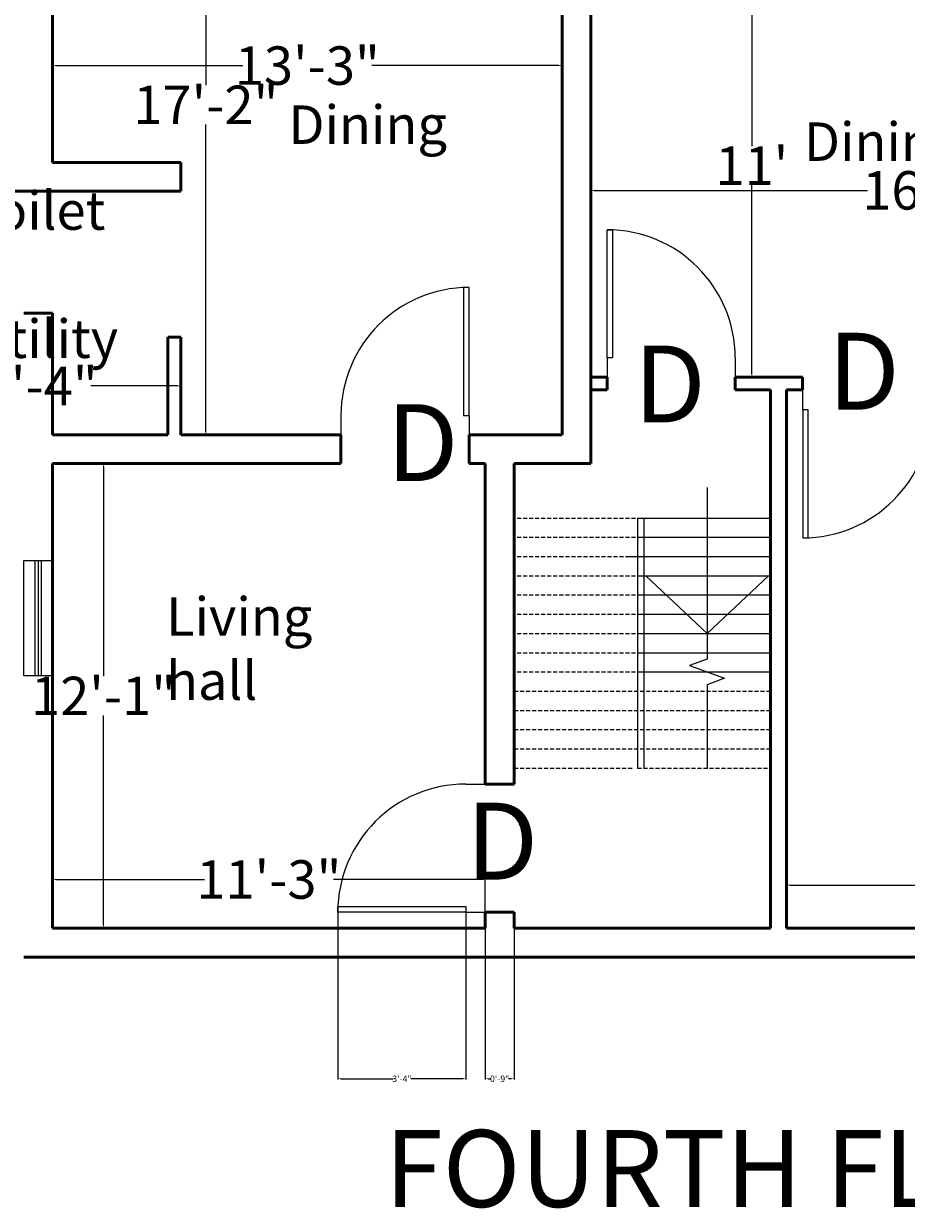
# Model space of a CAD drawing. Units: inches. Extents: x 409 to 7572, y 7 to 725.
# Tile 28 of 38: x 5677 to 5952, y 78 to 448. Entities that reach past the tile are written whole.
import ezdxf

# ---------------------------------------------------------------- set-up
doc = ezdxf.new("R2010")
doc.units = ezdxf.units.IN
doc.header["$MEASUREMENT"] = 0
doc.linetypes.add('HIDDEN', pattern=[0.375, 0.25, -0.125])
for name, color, linetype, lineweight in [('A-ANNO-DIMS', 2, 'Continuous', 18), ('A-ANNO-SYMB', 3, 'Continuous', 25), ('A-ANNO-TEXT', 7, 'Continuous', 35), ('A-AREA-IDEN', 7, 'Continuous', 25), ('A-DOOR', 3, 'Continuous', 25), ('A-FLOR-STRS', 6, 'Continuous', 25), ('A-FLOR-STRS-OVHD', 6, 'HIDDEN', 18), ('A-GLAZ', 4, 'Continuous', 25), ('A-WALL', 7, 'Continuous', 50)]:
    doc.layers.add(name, color=color, linetype=linetype, lineweight=lineweight)
doc.styles.get("Standard").update_dxf_attribs({"font": 'arial.ttf'})
doc.dimstyles.get("Standard").update_dxf_attribs({"dimtxt": 2, "dimasz": 1, "dimexe": 0.18, "dimexo": 0.0625, "dimgap": 0.09, "dimtad": 0, "dimtih": 1, "dimtoh": 1, "dimdec": 0, "dimzin": 0, "dimdsep": 46, "dimlunit": 3, "dimtxsty": 'Standard', "dimcen": 0.09, "dimadec": 0, "dimazin": 0, "dimtfac": 1, "dimtdec": 0, "dimtofl": 0, "dimtmove": 0, "dimatfit": 3, "dimfxl": 1, "dimtolj": 1, "dimtzin": 0, "dimarcsym": 0})

# ---------------------------------------------------------------- blocks, each defined once
blk = doc.blocks.new('*U2')
for p, q in [((0, 0), (0, -6)), ((-40, 0), (-40, -6))]:
    blk.add_line(p, q)
blk.add_lwpolyline([(0, 0), (0, 40), (-1.75, 40), (-1.75, 0)], close=True)
blk.add_arc((0, 0), 40, 90, 180)
blk = doc.blocks.new('*U3')
for p, q in [((0, 0), (0, -6)), ((40, 0), (40, -6))]:
    blk.add_line(p, q)
blk.add_lwpolyline([(0, 0), (0, 40), (1.75, 40), (1.75, 0)], close=True)
blk.add_arc((0, 0), 40, 0, 90)
blk = doc.blocks.new('*U4')
for p, q in [((0, 0), (0, -6)), ((40, 0), (40, -6))]:
    blk.add_line(p, q)
blk.add_lwpolyline([(0, 0), (0, 40), (1.75, 40), (1.75, 0)], close=True)
blk.add_arc((0, 0), 40, 0, 90)
blk = doc.blocks.new('*U5')
for p, q in [((0, 0), (0, 6)), ((40, 0), (40, 6))]:
    blk.add_line(p, q)
blk.add_lwpolyline([(0, 0), (0, -40), (1.75, -40), (1.75, 0)], close=True)
blk.add_arc((0, 0), 40, 270, 0)
blk = doc.blocks.new('*D124')
at = {"layer": 'A-ANNO-DIMS', "color": 0, "lineweight": -2, "transparency": 16777216}
for p, q in [((5914.78, 165.59), (5914.78, 179.18)), ((5915.78, 179), (5962.65, 179)), ((6049.78, 179), (6002.92, 179)), ((6050.78, 165.59), (6050.78, 179.18))]:
    blk.add_line(p, q, dxfattribs=at)
at = {"layer": 'A-ANNO-DIMS', "color": 0, "transparency": 16777216}
for points in [[(5915.78, 179.16), (5915.78, 178.83), (5914.78, 179)], [(6049.78, 179.16), (6049.78, 178.83), (6050.78, 179)]]:
    blk.add_solid(points, dxfattribs=at)
at = {"layer": 'DEFPOINTS', "color": 0, "transparency": 16777216}
for p in [(6050.78, 179), (5914.78, 165.53), (6050.78, 165.53)]:
    blk.add_point(p, dxfattribs=at)
at = {"layer": 'A-ANNO-DIMS', "color": 0, "transparency": 16777216, "insert": (5982.78, 179), "char_height": 2, "attachment_point": 5}
blk.add_mtext('\\A1;{\\H6x;11\'-4"}', dxfattribs=at)
blk = doc.blocks.new('*D125')
at = {"layer": 'A-ANNO-DIMS', "color": 0, "lineweight": -2, "transparency": 16777216}
for p, q in [((5685.78, 165.59), (5685.78, 180.91)), ((5686.78, 180.73), (5733.15, 180.73)), ((5819.78, 180.73), (5773.42, 180.73)), ((5820.78, 165.59), (5820.78, 180.91))]:
    blk.add_line(p, q, dxfattribs=at)
at = {"layer": 'A-ANNO-DIMS', "color": 0, "transparency": 16777216}
for points in [[(5686.78, 180.9), (5686.78, 180.56), (5685.78, 180.73)], [(5819.78, 180.9), (5819.78, 180.56), (5820.78, 180.73)]]:
    blk.add_solid(points, dxfattribs=at)
at = {"layer": 'DEFPOINTS', "color": 0, "transparency": 16777216}
for p in [(5820.78, 180.73), (5685.78, 165.53), (5820.78, 165.53)]:
    blk.add_point(p, dxfattribs=at)
at = {"layer": 'A-ANNO-DIMS', "color": 0, "transparency": 16777216, "insert": (5753.28, 180.73), "char_height": 2, "attachment_point": 5}
blk.add_mtext('\\A1;{\\H6x;11\'-3"}', dxfattribs=at)
blk = doc.blocks.new('*D126')
at = {"layer": 'A-ANNO-DIMS', "color": 0, "lineweight": -2, "transparency": 16777216}
for p, q in [((5685.85, 310.53), (5701.89, 310.53)), ((5701.71, 309.53), (5701.71, 244.15)), ((5701.71, 166.53), (5701.71, 231.92)), ((5685.85, 165.53), (5701.89, 165.53))]:
    blk.add_line(p, q, dxfattribs=at)
at = {"layer": 'A-ANNO-DIMS', "color": 0, "transparency": 16777216}
for points in [[(5701.54, 309.53), (5701.87, 309.53), (5701.71, 310.53)], [(5701.54, 166.53), (5701.87, 166.53), (5701.71, 165.53)]]:
    blk.add_solid(points, dxfattribs=at)
at = {"layer": 'DEFPOINTS', "color": 0, "transparency": 16777216}
for p in [(5685.78, 310.53), (5685.78, 165.53), (5701.71, 165.53)]:
    blk.add_point(p, dxfattribs=at)
at = {"layer": 'A-ANNO-DIMS', "color": 0, "transparency": 16777216, "insert": (5701.71, 238.03), "char_height": 2, "attachment_point": 5}
blk.add_mtext('\\A1;{\\H6x;12\'-1"}', dxfattribs=at)
blk = doc.blocks.new('*D138')
at = {"layer": 'A-ANNO-DIMS', "color": 0, "lineweight": -2, "transparency": 16777216}
for p, q in [((5685.78, 404.59), (5685.78, 434.95)), ((5686.78, 434.77), (5745.15, 434.77)), ((5843.78, 434.77), (5785.42, 434.77)), ((5844.78, 404.59), (5844.78, 434.95))]:
    blk.add_line(p, q, dxfattribs=at)
at = {"layer": 'A-ANNO-DIMS', "color": 0, "transparency": 16777216}
for points in [[(5686.78, 434.93), (5686.78, 434.6), (5685.78, 434.77)], [(5843.78, 434.93), (5843.78, 434.6), (5844.78, 434.77)]]:
    blk.add_solid(points, dxfattribs=at)
at = {"layer": 'DEFPOINTS', "color": 0, "transparency": 16777216}
for p in [(5844.78, 434.77), (5685.78, 404.53), (5844.78, 404.53)]:
    blk.add_point(p, dxfattribs=at)
at = {"layer": 'A-ANNO-DIMS', "color": 0, "transparency": 16777216, "insert": (5765.28, 434.77), "char_height": 2, "attachment_point": 5}
blk.add_mtext('\\A1;{\\H6x;13\'-3"}', dxfattribs=at)
blk = doc.blocks.new('*D139')
at = {"layer": 'A-ANNO-DIMS', "color": 0, "lineweight": -2, "transparency": 16777216}
for p, q in [((5742.72, 525.53), (5733.44, 525.53)), ((5733.62, 524.53), (5733.62, 428.65)), ((5733.62, 320.53), (5733.62, 416.42)), ((5750.72, 319.53), (5733.44, 319.53))]:
    blk.add_line(p, q, dxfattribs=at)
at = {"layer": 'A-ANNO-DIMS', "color": 0, "transparency": 16777216}
for points in [[(5733.45, 524.53), (5733.79, 524.53), (5733.62, 525.53)], [(5733.45, 320.53), (5733.79, 320.53), (5733.62, 319.53)]]:
    blk.add_solid(points, dxfattribs=at)
at = {"layer": 'DEFPOINTS', "color": 0, "transparency": 16777216}
for p in [(5742.78, 525.53), (5733.62, 319.53), (5750.78, 319.53)]:
    blk.add_point(p, dxfattribs=at)
at = {"layer": 'A-ANNO-DIMS', "color": 0, "transparency": 16777216, "insert": (5733.62, 422.53), "char_height": 2, "attachment_point": 5}
blk.add_mtext('\\A1;{\\H6x;17\'-2"}', dxfattribs=at)
blk = doc.blocks.new('*D136')
at = {"layer": 'A-ANNO-DIMS', "color": 0, "lineweight": -2, "transparency": 16777216}
for p, q in [((5853.78, 403.47), (5853.78, 395.65)), ((6045.78, 403.47), (6045.78, 395.65)), ((5854.78, 395.83), (5940.08, 395.83)), ((6044.78, 395.83), (5959.49, 395.83))]:
    blk.add_line(p, q, dxfattribs=at)
at = {"layer": 'A-ANNO-DIMS', "color": 0, "transparency": 16777216}
for points in [[(5854.78, 396), (5854.78, 395.66), (5853.78, 395.83)], [(6044.78, 396), (6044.78, 395.66), (6045.78, 395.83)]]:
    blk.add_solid(points, dxfattribs=at)
at = {"layer": 'DEFPOINTS', "color": 0, "transparency": 16777216}
for p in [(5853.78, 403.53), (6045.78, 403.53), (6045.78, 395.83)]:
    blk.add_point(p, dxfattribs=at)
at = {"layer": 'A-ANNO-DIMS', "color": 0, "transparency": 16777216, "insert": (5949.78, 395.83), "char_height": 2, "attachment_point": 5}
blk.add_mtext("\\A1;{\\H6x;16'}", dxfattribs=at)
blk = doc.blocks.new('*D140')
at = {"layer": 'A-ANNO-DIMS', "color": 0, "lineweight": -2, "transparency": 16777216}
for p, q in [((5908.05, 469.53), (5903.8, 469.53)), ((5903.98, 468.53), (5903.98, 409.65)), ((5903.98, 338.53), (5903.98, 397.42)), ((5909.22, 337.53), (5903.8, 337.53))]:
    blk.add_line(p, q, dxfattribs=at)
at = {"layer": 'A-ANNO-DIMS', "color": 0, "transparency": 16777216}
for points in [[(5903.81, 468.53), (5904.15, 468.53), (5903.98, 469.53)], [(5903.81, 338.53), (5904.15, 338.53), (5903.98, 337.53)]]:
    blk.add_solid(points, dxfattribs=at)
at = {"layer": 'DEFPOINTS', "color": 0, "transparency": 16777216}
for p in [(5908.11, 469.53), (5903.98, 337.53), (5909.28, 337.53)]:
    blk.add_point(p, dxfattribs=at)
at = {"layer": 'A-ANNO-DIMS', "color": 0, "transparency": 16777216, "insert": (5903.98, 403.53), "char_height": 2, "attachment_point": 5}
blk.add_mtext("\\A1;{\\H6x;11'}", dxfattribs=at)
blk = doc.blocks.new('*D145')
at = {"layer": 'A-ANNO-DIMS', "color": 0, "lineweight": -2, "transparency": 16777216}
for p, q in [((5637.78, 346.33), (5637.78, 334.6)), ((5725.78, 346.33), (5725.78, 334.6)), ((5638.78, 334.78), (5665.79, 334.78)), ((5724.78, 334.78), (5697.77, 334.78))]:
    blk.add_line(p, q, dxfattribs=at)
at = {"layer": 'A-ANNO-DIMS', "color": 0, "transparency": 16777216}
for points in [[(5638.78, 334.95), (5638.78, 334.61), (5637.78, 334.78)], [(5724.78, 334.95), (5724.78, 334.61), (5725.78, 334.78)]]:
    blk.add_solid(points, dxfattribs=at)
at = {"layer": 'DEFPOINTS', "color": 0, "transparency": 16777216}
for p in [(5637.78, 346.39), (5725.78, 346.39), (5725.78, 334.78)]:
    blk.add_point(p, dxfattribs=at)
at = {"layer": 'A-ANNO-DIMS', "color": 0, "transparency": 16777216, "insert": (5681.78, 334.78), "char_height": 2, "attachment_point": 5}
blk.add_mtext('\\A1;{\\H6x;7\'-4"}', dxfattribs=at)
blk = doc.blocks.new('WIN-36')
for p, q in [((1699.82, 514.65), (1699.82, 478.65)), ((1700.82, 514.65), (1700.82, 478.65)), ((1701.82, 514.65), (1701.82, 478.65))]:
    blk.add_line(p, q)
blk.add_lwpolyline([(1705.32, 514.65), (1705.32, 478.65), (1696.32, 478.65), (1696.32, 514.65)], close=True)
blk = doc.blocks.new('*D193')
at = {"layer": 'A-ANNO-DIMS', "color": 0, "lineweight": -2, "transparency": 16777216}
for p, q in [((5820.78, 165.47), (5820.78, 118.35)), ((5829.78, 165.47), (5829.78, 118.35)), ((5821.78, 118.53), (5822.54, 118.53)), ((5828.78, 118.53), (5828.03, 118.53))]:
    blk.add_line(p, q, dxfattribs=at)
at = {"layer": 'A-ANNO-DIMS', "color": 0, "transparency": 16777216}
for points in [[(5821.78, 118.7), (5821.78, 118.36), (5820.78, 118.53)], [(5828.78, 118.7), (5828.78, 118.36), (5829.78, 118.53)]]:
    blk.add_solid(points, dxfattribs=at)
at = {"layer": 'DEFPOINTS', "color": 0, "transparency": 16777216}
for p in [(5820.78, 165.53), (5829.78, 165.53), (5829.78, 118.53)]:
    blk.add_point(p, dxfattribs=at)
at = {"layer": 'A-ANNO-DIMS', "color": 0, "transparency": 16777216, "insert": (5825.28, 118.53), "char_height": 2, "attachment_point": 5}
blk.add_mtext('\\A1;0\'-9"', dxfattribs=at)
blk = doc.blocks.new('*D196')
at = {"layer": 'A-ANNO-DIMS', "color": 0, "lineweight": -2, "transparency": 16777216}
for p, q in [((5774.78, 170.47), (5774.78, 118.35)), ((5814.78, 170.47), (5814.78, 118.35)), ((5775.78, 118.53), (5792.04, 118.53)), ((5813.78, 118.53), (5797.53, 118.53))]:
    blk.add_line(p, q, dxfattribs=at)
at = {"layer": 'A-ANNO-DIMS', "color": 0, "transparency": 16777216}
for points in [[(5775.78, 118.7), (5775.78, 118.36), (5774.78, 118.53)], [(5813.78, 118.7), (5813.78, 118.36), (5814.78, 118.53)]]:
    blk.add_solid(points, dxfattribs=at)
at = {"layer": 'DEFPOINTS', "color": 0, "transparency": 16777216}
for p in [(5774.78, 170.53), (5814.78, 170.53), (5814.78, 118.53)]:
    blk.add_point(p, dxfattribs=at)
at = {"layer": 'A-ANNO-DIMS', "color": 0, "transparency": 16777216, "insert": (5794.78, 118.53), "char_height": 2, "attachment_point": 5}
blk.add_mtext('\\A1;3\'-4"', dxfattribs=at)

msp = doc.modelspace()

# ---------------------------------------------------------------- linework, layer by layer
at = {"layer": 'A-FLOR-STRS'}
for p, q in [((5889.99, 303.06), (5889.99, 257.53)), ((5868.28, 293.53), (5909.78, 293.53)), ((5868.28, 293.53), (5868.28, 215.53)), ((5870.28, 293.53), (5870.28, 215.53)), ((5868.28, 287.53), (5909.78, 287.53)), ((5865.44, 281.53), (5909.78, 281.53)), ((5868.28, 275.53), (5909.78, 275.53)), ((5889.99, 257.53), (5870.86, 275.53)), ((5889.99, 257.53), (5909.12, 275.53)), ((5868.28, 269.53), (5909.78, 269.53)), ((5868.28, 263.53), (5909.78, 263.53)), ((5868.28, 257.53), (5909.78, 257.53)), ((5868.28, 251.53), (5909.78, 251.53)), ((5868.28, 245.53), (5909.78, 245.53))]:
    msp.add_line(p, q, dxfattribs=at)
msp.add_lwpolyline([(5889.99, 257.71), (5889.99, 249.53), (5884.5, 247.53), (5895.49, 243.53), (5889.99, 241.53), (5889.99, 215.35)], dxfattribs=at)
at = {"layer": 'A-FLOR-STRS-OVHD', "ltscale": 5}
for p, q in [((5830.78, 293.53), (5868.28, 293.53)), ((5830.78, 287.53), (5868.28, 287.53)), ((5830.78, 281.53), (5865.44, 281.53)), ((5830.78, 275.53), (5868.28, 275.53)), ((5830.78, 269.53), (5868.28, 269.53)), ((5830.78, 263.53), (5868.28, 263.53)), ((5830.78, 257.53), (5868.28, 257.53)), ((5830.78, 251.53), (5868.28, 251.53)), ((5830.78, 245.53), (5868.28, 245.53)), ((5829.78, 239.53), (5909.78, 239.53)), ((5829.78, 233.53), (5909.78, 233.53)), ((5829.78, 227.53), (5909.78, 227.53)), ((5829.78, 221.53), (5909.78, 221.53)), ((5829.78, 215.53), (5867.28, 215.53)), ((5868.28, 215.53), (5909.78, 215.53))]:
    msp.add_line(p, q, dxfattribs=at)
at = {"layer": 'A-WALL'}
for p, q in [((5685.78, 525.53), (5685.78, 404.53)), ((5844.78, 525.53), (5844.78, 319.53)), ((5853.78, 469.53), (5853.78, 337.53)), ((5725.78, 404.53), (5685.78, 404.53)), ((5725.78, 404.53), (5725.78, 395.53)), ((5685.78, 395.53), (5637.78, 395.53)), ((5725.78, 395.53), (5685.78, 395.53)), ((5685.78, 357.53), (5676.78, 357.53)), ((5685.78, 357.53), (5685.78, 319.53)), ((5721.78, 350.03), (5721.78, 319.53)), ((5725.78, 350.03), (5721.78, 350.03)), ((5725.78, 350.03), (5725.78, 319.53)), ((5853.78, 337.53), (5858.78, 337.53)), ((5853.78, 337.53), (5853.78, 333.53)), ((5858.78, 337.53), (5858.78, 333.53)), ((5898.78, 337.53), (5919.78, 337.53)), ((5898.78, 337.53), (5898.78, 333.53)), ((5919.78, 333.53), (5919.78, 337.53)), ((5853.78, 333.53), (5858.78, 333.53)), ((5853.78, 333.53), (5853.78, 310.53)), ((5898.78, 333.53), (5909.78, 333.53)), ((5909.78, 333.53), (5909.78, 165.53)), ((5914.78, 333.53), (5919.78, 333.53)), ((5914.78, 333.53), (5914.78, 165.53)), ((5721.78, 319.53), (5685.78, 319.53)), ((5775.78, 319.53), (5725.78, 319.53)), ((5775.78, 319.53), (5775.78, 310.53)), ((5844.78, 319.53), (5815.78, 319.53)), ((5815.78, 310.53), (5815.78, 319.53)), ((5775.78, 310.53), (5685.78, 310.53)), ((5685.78, 310.53), (5685.78, 165.53)), ((5820.78, 310.53), (5815.78, 310.53)), ((5820.78, 310.53), (5820.78, 210.53)), ((5853.78, 310.53), (5829.78, 310.53)), ((5829.78, 310.53), (5829.78, 210.53)), ((5820.78, 210.53), (5829.78, 210.53)), ((5820.78, 170.53), (5820.78, 165.53)), ((5829.78, 170.53), (5820.78, 170.53)), ((5829.78, 170.53), (5829.78, 165.53)), ((5685.78, 165.53), (5820.78, 165.53)), ((5829.78, 165.53), (5909.78, 165.53)), ((5914.78, 165.53), (6050.78, 165.53)), ((5676.78, 156.53), (6050.78, 156.53))]:
    msp.add_line(p, q, dxfattribs=at)

# ---------------------------------------------------------------- block references
at = {"layer": 'A-DOOR'}
for name, p in [('*U4', (5858.78, 343.53)), ('*U2', (5815.78, 325.53)), ('*U5', (5919.84, 327.37))]:
    msp.add_blockref(name, p, dxfattribs=at)
at = {"layer": 'A-DOOR', "rotation": 90}
msp.add_blockref('*U3', (5814.78, 170.53), dxfattribs=at)
at = {"layer": 'A-GLAZ'}
msp.add_blockref('WIN-36', (3980.46, -234.38), dxfattribs=at)

# ---------------------------------------------------------------- texts
at = {"layer": 'A-ANNO-SYMB', "char_height": 24, "attachment_point": 1}
for insert in [(5927.61, 351.37), (5867.08, 347.4), (5789.92, 329.09), (5814.78, 204.69)]:
    msp.add_mtext_dynamic_manual_height_columns('D', width=19.1972, gutter_width=1, heights=[0], dxfattribs=dict(at, insert=insert))
at = {"layer": 'A-ANNO-TEXT', "insert": (5789.44, 102.52), "char_height": 24, "attachment_point": 1}
msp.add_mtext_dynamic_manual_height_columns('FOURTH FLOOR', width=577.2242, gutter_width=1, heights=[0], dxfattribs=at)
at = {"layer": 'A-AREA-IDEN', "char_height": 12, "attachment_point": 1}
for s, width, insert in [('Dining ', 67.5069, (5759.39, 422.33)), ('Dining ', 67.5069, (5920.22, 417.03)), ('toilet / utility', 49.2946, (5661.78, 395.53)), ('Living hall', 58.8843, (5721.21, 268.81))]:
    msp.add_mtext_dynamic_manual_height_columns(s, width=width, gutter_width=1, heights=[0], dxfattribs=dict(at, insert=insert))

# ---------------------------------------------------------------- dimensions: what is measured, and where the dimension line sits
at = {"layer": 'A-ANNO-DIMS'}
dim = msp.add_linear_dim(base=(5733.62, 319.53), p1=(5742.78, 525.53), p2=(5750.78, 319.53), angle=90, text='{\\H6x;<>}', dimstyle='Standard', override={"dimclrd": 0, "dimclre": 0, "dimclrt": 0}, dxfattribs=at)
dim.commit()
dim.dimension.update_dxf_attribs({"geometry": '*D139', "text_midpoint": (5733.62, 422.53), "dimtype": 160})
for base, p1, p2, picture, middle in [((5903.98, 337.53), (5908.11, 469.53), (5909.28, 337.53), '*D140', (5903.98, 403.53)), ((5701.71, 165.53), (5685.78, 310.53), (5685.78, 165.53), '*D126', (5701.71, 238.03))]:
    dim = msp.add_linear_dim(base=base, p1=p1, p2=p2, angle=90, text='{\\H6x;<>}', dimstyle='Standard', override={"dimclrd": 0, "dimclre": 0, "dimclrt": 0}, dxfattribs=at)
    dim.commit()
    dim.dimension.update_dxf_attribs({"geometry": picture, "text_midpoint": middle})
for base, p1, p2, picture, middle in [((5844.78, 434.77), (5685.78, 404.53), (5844.78, 404.53), '*D138', (5765.28, 434.77)), ((5725.78, 334.78), (5637.78, 346.39), (5725.78, 346.39), '*D145', (5681.78, 334.78)), ((5820.78, 180.73), (5685.78, 165.53), (5820.78, 165.53), '*D125', (5753.28, 180.73)), ((6050.78, 179), (5914.78, 165.53), (6050.78, 165.53), '*D124', (5982.78, 179))]:
    dim = msp.add_linear_dim(base=base, p1=p1, p2=p2, text='{\\H6x;<>}', dimstyle='Standard', override={"dimclrd": 0, "dimclre": 0, "dimclrt": 0}, dxfattribs=at)
    dim.commit()
    dim.dimension.update_dxf_attribs({"geometry": picture, "text_midpoint": middle})
dim = msp.add_linear_dim(base=(6045.78, 395.83), p1=(5853.78, 403.53), p2=(6045.78, 403.53), text='{\\H6x;<>}', dimstyle='Standard', override={"dimclrd": 0, "dimclre": 0, "dimclrt": 0}, dxfattribs=at)
dim.commit()
dim.dimension.update_dxf_attribs({"geometry": '*D136', "text_midpoint": (5949.78, 395.83), "dimtype": 160})
for base, p1, p2, picture, middle in [((5814.78, 118.53), (5774.78, 170.53), (5814.78, 170.53), '*D196', (5794.78, 118.53)), ((5829.78, 118.53), (5820.78, 165.53), (5829.78, 165.53), '*D193', (5825.28, 118.53))]:
    dim = msp.add_linear_dim(base=base, p1=p1, p2=p2, dimstyle='Standard', override={"dimdec": 1, "dimlfac": 1, "dimrnd": 0, "dimzin": 1, "dimdsep": 46, "dimlunit": 4, "dimfrac": 2}, dxfattribs=at)
    dim.commit()
    dim.dimension.update_dxf_attribs({"geometry": picture, "text_midpoint": middle})

doc.saveas('drawing.dxf')
